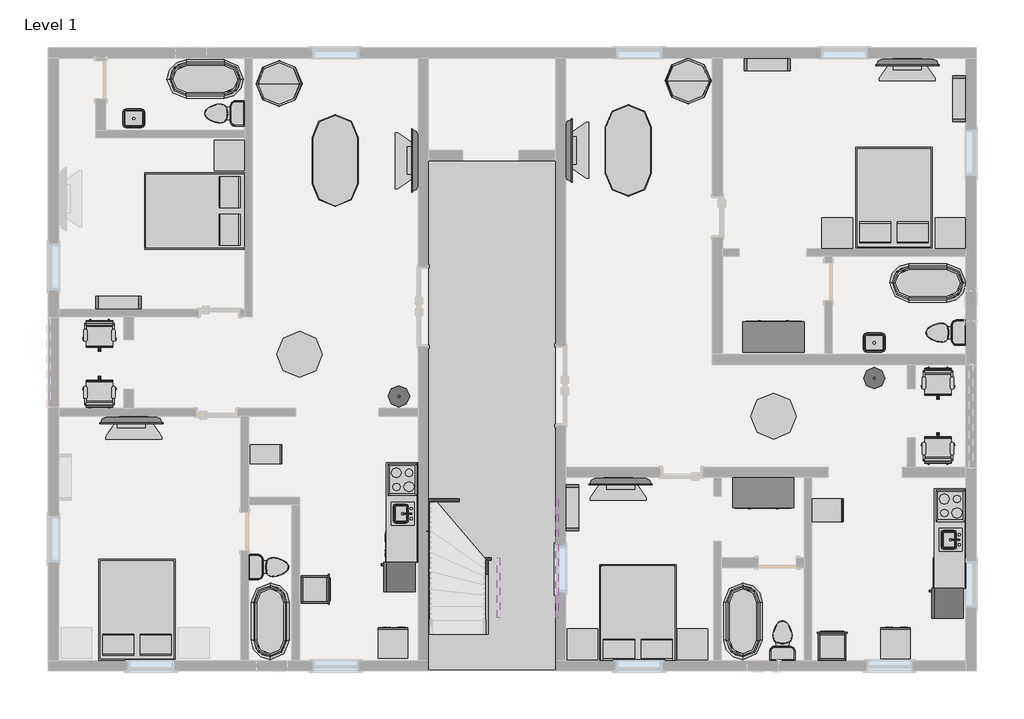
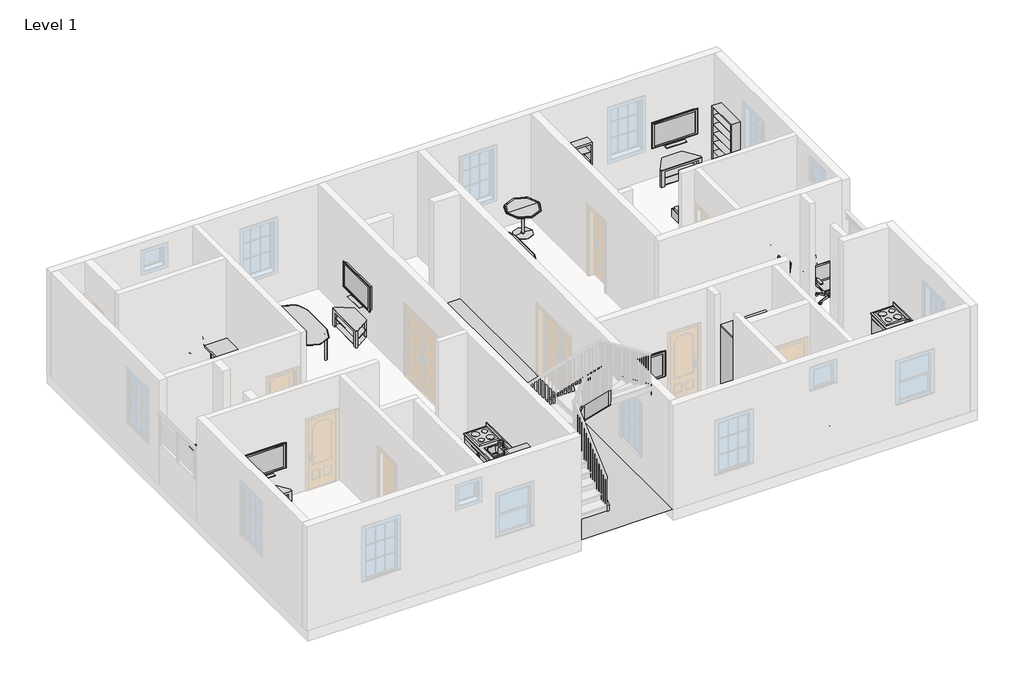
# One storey, part 4 of 4: 37 furniture elements, 15 proxies, 14 flow terminals, 8 members.
"""IFC4 building model written with IfcOpenShell, lengths in millimetres."""

from ifc_helpers import new_model, si_unit, frame, origin, place, context, project, spatial, polyline, outline, extrude, triangles, transform, mapped, element, save
from components import proxy_db4bb64d, proxy_7e1014cc, proxy_a6faaae8, proxy_53e5fb40, proxy_45b28599, kitchenette_medium_kitchenette_medium_844211aa, proxy_8b8c2dc4, proxy_c523a7b7, flow_terminal_871c2e40, flow_terminal_d49f872f, flow_terminal_62a433f7, toilet_domestic_3d_toilet_domestic_3d_f7549cf7, toilet_domestic_3d_toilet_domestic_3d_183bbd19, flow_terminal_b374fae2, furniture_1d2926bd, chair_task_arms_chair_task_arms_fa5a08ef, furniture_c6510c7c, furniture_9fa109b2, furniture_417d203a, furniture_fdf74506, tv_stand_tv_stand_6ce107e5, furniture_2c34a4f9, furniture_905aceb5, furniture_5bc9ed15, furniture_c80d6d9c

model = new_model("IFC4")

# Units and contexts
model_context = context("Model", 3, world=origin())
ifc_project = project(units=[si_unit("LENGTHUNIT", "METRE", prefix="MILLI")], contexts=[model_context])

# Site, building, storey
site = spatial("IfcSite", under=ifc_project)
building = spatial("IfcBuilding", under=site)
storey = spatial("IfcBuildingStorey", under=building, Name="Level 1", Elevation=0.0)

# Proxies
placement = place(None, origin())
element("IfcBuildingElementProxy", 1, Name="Building Element Proxy", at=placement, inside=storey, context=model_context, shape_type="Tessellation", body=[
    triangles([(-9093.3809967, 498.3923258, 0.0), (-6502.5809967, 498.3923258, 0.0), (-9093.3809967, 10671.0928345, 0.0), (-6502.5809967, 10671.0928345, 0.0)], [[3, 1, 4], [2, 4, 1]], closed=False),
])
proxy_shape = proxy_db4bb64d(model_context)
element("IfcBuildingElementProxy", 2, Name="15\" x 24\" x 34 1/2\"", ObjectType="15\" x 24\" x 34 1/2\"", at=placement, inside=storey, context=model_context, shape_type="MappedRepresentation", body=[
    mapped(proxy_shape, transform((-12040.0313324, 4522.9748669, 0.0), x_axis=(0.0, 1.000000000000001, 0.0), y_axis=(-1.000000000000001, 0.0, 0.0), z_axis=(0.0, 0.0, 1.0))),
])
proxy_2_shape = proxy_7e1014cc(model_context)
element("IfcBuildingElementProxy", 3, Name="18\" x 24\" x 34 1/2\"", ObjectType="18\" x 24\" x 34 1/2\"", at=placement, inside=storey, context=model_context, shape_type="MappedRepresentation", body=[
    mapped(proxy_2_shape, transform((-851.3313324, 3367.2748669, 0.0), x_axis=(0.0, 1.000000000000001, 0.0), y_axis=(-1.000000000000001, 0.0, 0.0), z_axis=(0.0, 0.0, 1.0))),
])
proxy_3_shape = proxy_a6faaae8(model_context)
element("IfcBuildingElementProxy", 4, Name="Cook Top-4 Unit2 : 22\" x 20\"", ObjectType="Cook Top-4 Unit2 : 22\" x 20\"", at=placement, inside=storey, context=model_context, shape_type="MappedRepresentation", body=[
    mapped(proxy_3_shape, transform((-9575.9808972, 4282.9923354, 0.0), x_axis=(0.0, -1.0000000000000004, 0.0), y_axis=(1.0000000000000004, 0.0, 0.0), z_axis=(0.0, 0.0, 1.0))),
])
element("IfcBuildingElementProxy", 5, Name="Cook Top-4 Unit2 : 22\" x 20\"", ObjectType="Cook Top-4 Unit2 : 22\" x 20\"", at=placement, inside=storey, context=model_context, shape_type="MappedRepresentation", body=[
    mapped(proxy_3_shape, transform((1346.0191028, 3762.2923354, 0.0), x_axis=(0.0, -1.0, 0.0), y_axis=(1.0, 0.0, 0.0), z_axis=(0.0, 0.0, 1.0))),
])
proxy_4_shape = proxy_53e5fb40(model_context)
element("IfcBuildingElementProxy", 6, Name="Dishwasher : 23\" x 23 11/16\" x 33 1/2\"", ObjectType="Dishwasher : 23\" x 23 11/16\" x 33 1/2\"", at=placement, inside=storey, context=model_context, shape_type="MappedRepresentation", body=[
    mapped(proxy_4_shape, transform((-9398.1808972, 1285.7923354, 0.0), x_axis=(-1.0000000000000013, 0.0, 0.0), y_axis=(0.0, -1.0000000000000013, 0.0), z_axis=(0.0, 0.0, 1.0))),
])
element("IfcBuildingElementProxy", 7, Name="Dishwasher : 23\" x 23 11/16\" x 33 1/2\"", ObjectType="Dishwasher : 23\" x 23 11/16\" x 33 1/2\"", at=placement, inside=storey, context=model_context, shape_type="MappedRepresentation", body=[
    mapped(proxy_4_shape, transform((613.9311676, 1284.4748669, 0.0), x_axis=(-1.0000000000000004, 0.0, 0.0), y_axis=(0.0, -1.0000000000000004, 0.0), z_axis=(0.0, 0.0, 1.0))),
])
proxy_5_shape = proxy_45b28599(model_context)
element("IfcBuildingElementProxy", 8, Name="Dishwasher : 24\" x 24\" x 34\"", ObjectType="Dishwasher : 24\" x 24\" x 34\"", at=placement, inside=storey, context=model_context, shape_type="MappedRepresentation", body=[
    mapped(proxy_5_shape, transform((-9867.830462, 3331.8098039, 0.0), x_axis=(0.0, -1.0000000000000004, 0.0), y_axis=(1.0000000000000004, 0.0, 0.0), z_axis=(0.0, 0.0, 1.0))),
])
element("IfcBuildingElementProxy", 9, Name="Dishwasher : 24\" x 24\" x 34\"", ObjectType="Dishwasher : 24\" x 24\" x 34\"", at=placement, inside=storey, context=model_context, shape_type="MappedRepresentation", body=[
    mapped(proxy_5_shape, transform((1054.169538, 2811.1098039, 0.0), x_axis=(0.0, -1.0, 0.0), y_axis=(1.0, 0.0, 0.0), z_axis=(0.0, 0.0, 1.0))),
])
kitchenette_medium_kitchenette_medium_shape = kitchenette_medium_kitchenette_medium_844211aa(model_context)
element("IfcBuildingElementProxy", 10, Name="Kitchenette - Medium : Kitchenette - Medium", ObjectType="Kitchenette - Medium : Kitchenette - Medium", at=placement, inside=storey, context=model_context, shape_type="MappedRepresentation", body=[
    mapped(kitchenette_medium_kitchenette_medium_shape, transform((-9271.1808972, 3958.8300403, 0.0), x_axis=(0.0, -1.0000000000000004, 0.0), y_axis=(1.0000000000000004, 0.0, 0.0), z_axis=(0.0, 0.0, 1.0))),
])
element("IfcBuildingElementProxy", 11, Name="Kitchenette - Medium : Kitchenette - Medium", ObjectType="Kitchenette - Medium : Kitchenette - Medium", at=placement, inside=storey, context=model_context, shape_type="MappedRepresentation", body=[
    mapped(kitchenette_medium_kitchenette_medium_shape, transform((1650.8191028, 3438.1300403, 0.0), x_axis=(0.0, -1.0, 0.0), y_axis=(1.0, 0.0, 0.0), z_axis=(0.0, 0.0, 1.0))),
])
proxy_6_shape = proxy_8b8c2dc4(model_context)
element("IfcBuildingElementProxy", 12, Name="Oven Double-Built-in : 21 1/2\" x 39 1/4\" x 21\"", ObjectType="Oven Double-Built-in : 21 1/2\" x 39 1/4\" x 21\"", at=placement, inside=storey, context=model_context, shape_type="MappedRepresentation", body=[
    mapped(proxy_6_shape, transform((-1051.3558245, 1096.6581944, 0.0), x_axis=(-1.0000000000000002, 0.0, 0.0), y_axis=(0.0, -1.0000000000000002, 0.0), z_axis=(0.0, 0.0, 1.0))),
])
element("IfcBuildingElementProxy", 13, Name="Oven Double-Built-in : 21 1/2\" x 39 1/4\" x 21\"", ObjectType="Oven Double-Built-in : 21 1/2\" x 39 1/4\" x 21\"", at=placement, inside=storey, context=model_context, shape_type="MappedRepresentation", body=[
    mapped(proxy_6_shape, transform((-11187.5150383, 2133.7672627, 0.0), x_axis=(0.0, 1.0000000000000002, 0.0), y_axis=(-1.0000000000000002, 0.0, 0.0), z_axis=(0.0, 0.0, 1.0))),
])
proxy_7_shape = proxy_c523a7b7(model_context)
element("IfcBuildingElementProxy", 14, Name="Refrigerator : 24\" x 25\" LH", ObjectType="Refrigerator : 24\" x 25\" LH", at=placement, inside=storey, context=model_context, shape_type="MappedRepresentation", body=[
    mapped(proxy_7_shape, transform((-9621.6298687, 2346.2423354, 0.0), x_axis=(0.0, -1.0000000000000004, 0.0), y_axis=(1.0000000000000004, 0.0, 0.0), z_axis=(0.0, 0.0, 1.0))),
])
element("IfcBuildingElementProxy", 15, Name="Refrigerator : 24\" x 25\" LH", ObjectType="Refrigerator : 24\" x 25\" LH", at=placement, inside=storey, context=model_context, shape_type="MappedRepresentation", body=[
    mapped(proxy_7_shape, transform((1300.3701313, 1825.5423354, 0.0), x_axis=(0.0, -1.0, 0.0), y_axis=(1.0, 0.0, 0.0), z_axis=(0.0, 0.0, 1.0))),
])

# Flow terminals
flow_terminal_shape = flow_terminal_871c2e40(model_context)
element("IfcFlowTerminal", 16, ObjectType="Sink Kitchen-Island : 18\" x 18\"", at=placement, inside=storey, context=model_context, shape_type="MappedRepresentation", body=[
    mapped(flow_terminal_shape, transform((-9578.3262983, 3625.581576, -14.4), x_axis=(0.0, -1.0000000000000004, 0.0), y_axis=(1.0000000000000004, 0.0, 0.0), z_axis=(0.0, 0.0, 1.0))),
])
element("IfcFlowTerminal", 17, ObjectType="Sink Kitchen-Island : 18\" x 18\"", at=placement, inside=storey, context=model_context, shape_type="MappedRepresentation", body=[
    mapped(flow_terminal_shape, transform((1343.6737017, 3104.881576, -14.4), x_axis=(0.0, -1.0, 0.0), y_axis=(1.0, 0.0, 0.0), z_axis=(0.0, 0.0, 1.0))),
])
flow_terminal_2_shape = flow_terminal_d49f872f(model_context)
element("IfcFlowTerminal", 18, ObjectType="Sink Vanity-Round : 19\" x 19\"", at=placement, inside=storey, context=model_context, shape_type="MappedRepresentation", body=[
    mapped(flow_terminal_2_shape, transform((-274.6326378, 6226.604818, 609.6), x_axis=(1.0, 0.0, 0.0), y_axis=(0.0, 1.0, 0.0), z_axis=(0.0, 0.0, 1.0))),
])
element("IfcFlowTerminal", 19, ObjectType="Sink Vanity-Round : 19\" x 19\"", at=placement, inside=storey, context=model_context, shape_type="MappedRepresentation", body=[
    mapped(flow_terminal_2_shape, transform((-9555.5291566, 6031.4364541, 609.6), x_axis=(-1.0000000000000004, 0.0, 0.0), y_axis=(0.0, -1.0000000000000004, 0.0), z_axis=(0.0, 0.0, 1.0))),
])
flow_terminal_3_shape = flow_terminal_62a433f7(model_context)
element("IfcFlowTerminal", 20, ObjectType="Sink Vanity-Square : 20\" x 18\"", at=placement, inside=storey, context=model_context, shape_type="MappedRepresentation", body=[
    mapped(flow_terminal_3_shape, transform((-162.2916566, 6965.0377365, 609.6), x_axis=(-1.0000000000000004, 0.0, 0.0), y_axis=(0.0, -1.0000000000000004, 0.0), z_axis=(0.0, 0.0, 1.0))),
])
element("IfcFlowTerminal", 21, ObjectType="Sink Vanity-Square : 20\" x 18\"", at=placement, inside=storey, context=model_context, shape_type="MappedRepresentation", body=[
    mapped(flow_terminal_3_shape, transform((-14919.6916566, 11435.4377365, 609.6), x_axis=(-1.0, 0.0, 0.0), y_axis=(0.0, -1.0, 0.0), z_axis=(0.0, 0.0, 1.0))),
])
toilet_domestic_3d_toilet_domestic_3d_shape = toilet_domestic_3d_toilet_domestic_3d_f7549cf7(model_context)
toilet_domestic_3d_toilet_domestic_3d_2_shape = toilet_domestic_3d_toilet_domestic_3d_183bbd19(model_context)
element("IfcFlowTerminal", 22, ObjectType="Toilet-Domestic-3D : Toilet-Domestic-3D", at=placement, inside=storey, context=model_context, shape_type="MappedRepresentation", body=[
    mapped(toilet_domestic_3d_toilet_domestic_3d_shape, transform((-12154.6848699, 2543.0923354, 0.0), x_axis=(0.0, 1.0000000000000002, 0.0), y_axis=(-1.0000000000000002, 0.0, 0.0), z_axis=(0.0, 0.0, 1.0))),
    mapped(toilet_domestic_3d_toilet_domestic_3d_2_shape, transform((-12154.6848699, 2543.0923354, 0.0), x_axis=(0.0, 1.0000000000000002, 0.0), y_axis=(-1.0000000000000002, 0.0, 0.0), z_axis=(0.0, 0.0, 1.0))),
])
element("IfcFlowTerminal", 23, ObjectType="Toilet-Domestic-3D : Toilet-Domestic-3D", at=placement, inside=storey, context=model_context, shape_type="MappedRepresentation", body=[
    mapped(toilet_domestic_3d_toilet_domestic_3d_shape, transform((-2006.7808972, 1170.8883628, 0.0), x_axis=(-1.0000000000000004, 0.0, 0.0), y_axis=(0.0, -1.0000000000000004, 0.0), z_axis=(0.0, 0.0, 1.0))),
    mapped(toilet_domestic_3d_toilet_domestic_3d_2_shape, transform((-2006.7808972, 1170.8883628, 0.0), x_axis=(-1.0000000000000004, 0.0, 0.0), y_axis=(0.0, -1.0000000000000004, 0.0), z_axis=(0.0, 0.0, 1.0))),
])
element("IfcFlowTerminal", 24, ObjectType="Toilet-Domestic-3D : Toilet-Domestic-3D", at=placement, inside=storey, context=model_context, shape_type="MappedRepresentation", body=[
    mapped(toilet_domestic_3d_toilet_domestic_3d_shape, transform((1156.1230754, 7216.6923354, 0.0), x_axis=(0.0, -1.0000000000000002, 0.0), y_axis=(1.0000000000000002, 0.0, 0.0), z_axis=(0.0, 0.0, 1.0))),
    mapped(toilet_domestic_3d_toilet_domestic_3d_2_shape, transform((1156.1230754, 7216.6923354, 0.0), x_axis=(0.0, -1.0000000000000002, 0.0), y_axis=(1.0000000000000002, 0.0, 0.0), z_axis=(0.0, 0.0, 1.0))),
])
element("IfcFlowTerminal", 25, ObjectType="Toilet-Domestic-3D : Toilet-Domestic-3D", at=placement, inside=storey, context=model_context, shape_type="MappedRepresentation", body=[
    mapped(toilet_domestic_3d_toilet_domestic_3d_shape, transform((-13220.2769246, 11585.4923354, 0.0), x_axis=(0.0, -1.0, 0.0), y_axis=(1.0, 0.0, 0.0), z_axis=(0.0, 0.0, 1.0))),
    mapped(toilet_domestic_3d_toilet_domestic_3d_2_shape, transform((-13220.2769246, 11585.4923354, 0.0), x_axis=(0.0, -1.0, 0.0), y_axis=(1.0, 0.0, 0.0), z_axis=(0.0, 0.0, 1.0))),
])
flow_terminal_4_shape = flow_terminal_b374fae2(model_context)
element("IfcFlowTerminal", 26, ObjectType="Tub-Free Standing-3D : 30\" x 60\"", at=placement, inside=storey, context=model_context, shape_type="MappedRepresentation", body=[
    mapped(flow_terminal_4_shape, transform((888.8191028, 8207.2923354, 0.0), x_axis=(0.0, -1.0000000000000002, 0.0), y_axis=(1.0000000000000002, 0.0, 0.0), z_axis=(0.0, 0.0, 1.0))),
])
element("IfcFlowTerminal", 27, ObjectType="Tub-Free Standing-3D : 30\" x 60\"", at=placement, inside=storey, context=model_context, shape_type="MappedRepresentation", body=[
    mapped(flow_terminal_4_shape, transform((-2794.1808972, 1463.5923354, 0.0), x_axis=(-1.0000000000000004, 0.0, 0.0), y_axis=(0.0, -1.0000000000000004, 0.0), z_axis=(0.0, 0.0, 1.0))),
])
element("IfcFlowTerminal", 28, ObjectType="Tub-Free Standing-3D : 30\" x 60\"", at=placement, inside=storey, context=model_context, shape_type="MappedRepresentation", body=[
    mapped(flow_terminal_4_shape, transform((-13512.9808972, 12271.2923354, 0.0), x_axis=(0.0, -1.0, 0.0), y_axis=(1.0, 0.0, 0.0), z_axis=(0.0, 0.0, 1.0))),
])
element("IfcFlowTerminal", 29, ObjectType="Tub-Free Standing-3D : 30\" x 60\"", at=placement, inside=storey, context=model_context, shape_type="MappedRepresentation", body=[
    mapped(flow_terminal_4_shape, transform((-12217.5808972, 1463.5923354, 0.0), x_axis=(-0.9999999999999998, 0.0, 0.0), y_axis=(0.0, -0.9999999999999998, 0.0), z_axis=(0.0, 0.0, 1.0))),
])

# Furniture
furniture_shape = furniture_1d2926bd(model_context)
element("IfcFurniture", 30, ObjectType="Bed-Box : Queen 60\" x 79\"", at=placement, inside=storey, context=model_context, shape_type="MappedRepresentation", body=[
    mapped(furniture_shape, transform((-13481.751389, 9981.5447944, 0.0), x_axis=(0.0, -1.0000000000000002, 0.0), y_axis=(1.0000000000000002, 0.0, 0.0), z_axis=(0.0, 0.0, 1.0))),
])
element("IfcFurniture", 31, ObjectType="Bed-Box : Queen 60\" x 79\"", at=placement, inside=storey, context=model_context, shape_type="MappedRepresentation", body=[
    mapped(furniture_shape, transform((-14532.7284382, 1457.7628272, 0.0), x_axis=(-0.9999999999999998, 0.0, 0.0), y_axis=(0.0, -0.9999999999999998, 0.0), z_axis=(0.0, 0.0, 1.0))),
])
element("IfcFurniture", 32, ObjectType="Bed-Box : Queen 60\" x 79\"", at=placement, inside=storey, context=model_context, shape_type="MappedRepresentation", body=[
    mapped(furniture_shape, transform((-4550.5284382, 1356.1628272, 0.0), x_axis=(-1.0, 0.0, 0.0), y_axis=(0.0, -1.0, 0.0), z_axis=(0.0, 0.0, 1.0))),
])
element("IfcFurniture", 33, ObjectType="Bed-Box : Queen 60\" x 79\"", at=placement, inside=storey, context=model_context, shape_type="MappedRepresentation", body=[
    mapped(furniture_shape, transform((554.8715618, 9674.6628272, 0.0), x_axis=(-1.0, 0.0, 0.0), y_axis=(0.0, -1.0, 0.0), z_axis=(0.0, 0.0, 1.0))),
])
chair_task_arms_chair_task_arms_shape = chair_task_arms_chair_task_arms_fa5a08ef(model_context)
element("IfcFurniture", 34, ObjectType="Chair-Task Arms : Chair-Task Arms", at=placement, inside=storey, context=model_context, shape_type="MappedRepresentation", body=[
    mapped(chair_task_arms_chair_task_arms_shape, transform((-15762.1717169, 5978.5464338, 0.0), x_axis=(1.0, 0.0, 0.0), y_axis=(0.0, 1.0, 0.0), z_axis=(0.0, 0.0, 1.0))),
])
element("IfcFurniture", 35, ObjectType="Chair-Task Arms : Chair-Task Arms", at=placement, inside=storey, context=model_context, shape_type="MappedRepresentation", body=[
    mapped(chair_task_arms_chair_task_arms_shape, transform((-15480.1900775, 7210.2382371, 0.0), x_axis=(-1.0000000000000004, 0.0, 0.0), y_axis=(0.0, -1.0000000000000004, 0.0), z_axis=(0.0, 0.0, 1.0))),
])
element("IfcFurniture", 36, ObjectType="Chair-Task Arms : Chair-Task Arms", at=placement, inside=storey, context=model_context, shape_type="MappedRepresentation", body=[
    mapped(chair_task_arms_chair_task_arms_shape, transform((1233.0099225, 6257.7382371, 0.0), x_axis=(-1.0, 0.0, 0.0), y_axis=(0.0, -1.0, 0.0), z_axis=(0.0, 0.0, 1.0))),
])
element("IfcFurniture", 37, ObjectType="Chair-Task Arms : Chair-Task Arms", at=placement, inside=storey, context=model_context, shape_type="MappedRepresentation", body=[
    mapped(chair_task_arms_chair_task_arms_shape, transform((951.0282831, 4860.9464338, 0.0), x_axis=(1.0000000000000002, 0.0, 0.0), y_axis=(0.0, 1.0000000000000002, 0.0), z_axis=(0.0, 0.0, 1.0))),
])
furniture_2_shape = furniture_c6510c7c(model_context)
element("IfcFurniture", 38, ObjectType="Counter Top w Sink Hole : 24\" Depth", at=placement, inside=storey, context=model_context, shape_type="MappedRepresentation", body=[
    mapped(furniture_2_shape, transform((-9271.1808972, 3425.4300403, -14.4), x_axis=(0.0, -1.0000000000000004, 0.0), y_axis=(1.0000000000000004, 0.0, 0.0), z_axis=(0.0, 0.0, 1.0))),
])
element("IfcFurniture", 39, ObjectType="Counter Top w Sink Hole : 24\" Depth", at=placement, inside=storey, context=model_context, shape_type="MappedRepresentation", body=[
    mapped(furniture_2_shape, transform((1650.8191028, 2904.7300403, -14.4), x_axis=(0.0, -1.0, 0.0), y_axis=(1.0, 0.0, 0.0), z_axis=(0.0, 0.0, 1.0))),
])
furniture_3_shape = furniture_9fa109b2(model_context)
element("IfcFurniture", 40, ObjectType="Dresser : 48\" x 72\" x 24\"", at=placement, inside=storey, context=model_context, shape_type="MappedRepresentation", body=[
    mapped(furniture_3_shape, transform((-2453.774157, 6764.6293813, 0.0), x_axis=(-1.0000000000000004, 0.0, 0.0), y_axis=(0.0, -1.0000000000000004, 0.0), z_axis=(0.0, 0.0, 1.0))),
])
element("IfcFurniture", 41, ObjectType="Dresser : 48\" x 72\" x 24\"", at=placement, inside=storey, context=model_context, shape_type="MappedRepresentation", body=[
    mapped(furniture_3_shape, transform((-2118.5876374, 4392.1552895, 0.0), x_axis=(1.0, 0.0, 0.0), y_axis=(0.0, 1.0, 0.0), z_axis=(0.0, 0.0, 1.0))),
])
furniture_4_shape = furniture_417d203a(model_context)
element("IfcFurniture", 42, ObjectType="Shelving : 36\" x 10\" x 72\"", at=placement, inside=storey, context=model_context, shape_type="MappedRepresentation", body=[
    mapped(furniture_4_shape, transform((-15240.1808972, 8118.3923354, 0.0), x_axis=(1.0, 0.0, 0.0), y_axis=(0.0, 1.0, 0.0), z_axis=(0.0, 0.0, 1.0))),
])
element("IfcFurniture", 43, ObjectType="Shelving : 36\" x 10\" x 72\"", at=placement, inside=storey, context=model_context, shape_type="MappedRepresentation", body=[
    mapped(furniture_4_shape, transform((-6502.5808972, 3724.1923354, 0.0), x_axis=(0.0, 1.0000000000000002, 0.0), y_axis=(-1.0000000000000002, 0.0, 0.0), z_axis=(0.0, 0.0, 1.0))),
])
element("IfcFurniture", 44, ObjectType="Shelving : 36\" x 10\" x 72\"", at=placement, inside=storey, context=model_context, shape_type="MappedRepresentation", body=[
    mapped(furniture_4_shape, transform((-2311.5808972, 12258.5923354, 0.0), x_axis=(-1.0000000000000004, 0.0, 0.0), y_axis=(0.0, -1.0000000000000004, 0.0), z_axis=(0.0, 0.0, 1.0))),
])
element("IfcFurniture", 45, ObjectType="Shelving : 36\" x 10\" x 72\"", at=placement, inside=storey, context=model_context, shape_type="MappedRepresentation", body=[
    mapped(furniture_4_shape, transform((1815.9191028, 11877.5923354, 0.0), x_axis=(0.0, -1.0000000000000002, 0.0), y_axis=(1.0000000000000002, 0.0, 0.0), z_axis=(0.0, 0.0, 1.0))),
])
furniture_5_shape = furniture_fdf74506(model_context)
element("IfcFurniture", 46, ObjectType="TV - Flat Screen : 50\"", at=placement, inside=storey, context=model_context, shape_type="MappedRepresentation", body=[
    mapped(furniture_5_shape, transform((-14982.2363831, 5470.9664028, 914.4), x_axis=(1.0, 0.0, 0.0), y_axis=(0.0, 1.0, 0.0), z_axis=(0.0, 0.0, 1.0))),
])
element("IfcFurniture", 47, ObjectType="TV - Flat Screen : 50\"", at=placement, inside=storey, context=model_context, shape_type="MappedRepresentation", body=[
    mapped(furniture_5_shape, transform((-5228.6363831, 4251.4680978, 914.4), x_axis=(1.0, 0.0, 0.0), y_axis=(0.0, 1.0, 0.0), z_axis=(0.0, 0.0, 1.0))),
])
element("IfcFurniture", 48, ObjectType="TV - Flat Screen : 50\"", at=placement, inside=storey, context=model_context, shape_type="MappedRepresentation", body=[
    mapped(furniture_5_shape, transform((486.3636169, 12605.0152005, 914.4), x_axis=(1.0, 0.0, 0.0), y_axis=(0.0, 1.0, 0.0), z_axis=(0.0, 0.0, 1.0))),
])
element("IfcFurniture", 49, ObjectType="TV - Flat Screen : 50\"", at=placement, inside=storey, context=model_context, shape_type="MappedRepresentation", body=[
    mapped(furniture_5_shape, transform((-9329.7195209, 10641.7478213, 914.4), x_axis=(0.0, -0.9999999999999998, 0.0), y_axis=(0.9999999999999998, 0.0, 0.0), z_axis=(0.0, 0.0, 1.0))),
])
element("IfcFurniture", 50, ObjectType="TV - Flat Screen : 50\"", at=placement, inside=storey, context=model_context, shape_type="MappedRepresentation", body=[
    mapped(furniture_5_shape, transform((-6266.2422736, 10852.8368496, 914.4), x_axis=(0.0, 1.0000000000000004, 0.0), y_axis=(-1.0000000000000004, 0.0, 0.0), z_axis=(0.0, 0.0, 1.0))),
])
tv_stand_tv_stand_shape = tv_stand_tv_stand_6ce107e5(model_context)
element("IfcFurniture", 51, ObjectType="TV Stand : TV Stand", at=placement, inside=storey, context=model_context, shape_type="MappedRepresentation", body=[
    mapped(tv_stand_tv_stand_shape, transform((357.2311007, 12690.3923354, 0.0), x_axis=(1.0, 0.0, 0.0), y_axis=(0.0, 1.0, 0.0), z_axis=(0.0, 0.0, 1.0))),
])
element("IfcFurniture", 52, ObjectType="TV Stand : TV Stand", at=placement, inside=storey, context=model_context, shape_type="MappedRepresentation", body=[
    mapped(tv_stand_tv_stand_shape, transform((-15060.5688993, 5552.9923354, 0.0), x_axis=(1.0, 0.0, 0.0), y_axis=(0.0, 1.0, 0.0), z_axis=(0.0, 0.0, 1.0))),
])
element("IfcFurniture", 53, ObjectType="TV Stand : TV Stand", at=placement, inside=storey, context=model_context, shape_type="MappedRepresentation", body=[
    mapped(tv_stand_tv_stand_shape, transform((-5408.5688993, 4333.7923354, 0.0), x_axis=(1.0, 0.0, 0.0), y_axis=(0.0, 1.0, 0.0), z_axis=(0.0, 0.0, 1.0))),
])
element("IfcFurniture", 54, ObjectType="TV Stand : TV Stand", at=placement, inside=storey, context=model_context, shape_type="MappedRepresentation", body=[
    mapped(tv_stand_tv_stand_shape, transform((-6324.7808972, 10723.7043334, 0.0), x_axis=(0.0, 1.0, 0.0), y_axis=(-1.0, 0.0, 0.0), z_axis=(0.0, 0.0, 1.0))),
])
element("IfcFurniture", 55, ObjectType="TV Stand : TV Stand", at=placement, inside=storey, context=model_context, shape_type="MappedRepresentation", body=[
    mapped(tv_stand_tv_stand_shape, transform((-9271.1808972, 10770.8803375, 0.0), x_axis=(0.0, -1.0000000000000002, 0.0), y_axis=(1.0000000000000002, 0.0, 0.0), z_axis=(0.0, 0.0, 1.0))),
])
furniture_6_shape = furniture_2c34a4f9(model_context)
element("IfcFurniture", 56, ObjectType="Table-Dining Oval : 36\" x 72\"", at=placement, inside=storey, context=model_context, shape_type="MappedRepresentation", body=[
    mapped(furniture_6_shape, transform((-5438.2792579, 11250.7120076, 0.0), x_axis=(0.0, 1.0, 0.0), y_axis=(-1.0, 0.0, 0.0), z_axis=(0.0, 0.0, 1.0))),
])
element("IfcFurniture", 57, ObjectType="Table-Dining Oval : 36\" x 72\"", at=placement, inside=storey, context=model_context, shape_type="MappedRepresentation", body=[
    mapped(furniture_6_shape, transform((-11280.2792579, 11047.5120076, 0.0), x_axis=(0.0, 1.0, 0.0), y_axis=(-1.0, 0.0, 0.0), z_axis=(0.0, 0.0, 1.0))),
])
furniture_7_shape = furniture_905aceb5(model_context)
element("IfcFurniture", 58, ObjectType="Table-Dining Round w Chairs : 36\" Diameter", at=placement, inside=storey, context=model_context, shape_type="MappedRepresentation", body=[
    mapped(furniture_7_shape, transform((-2288.2628644, 5737.8710239, 0.0), x_axis=(1.0, 0.0, 0.0), y_axis=(0.0, 1.0, 0.0), z_axis=(0.0, 0.0, 1.0))),
])
element("IfcFurniture", 59, ObjectType="Table-Dining Round w Chairs : 36\" Diameter", at=placement, inside=storey, context=model_context, shape_type="MappedRepresentation", body=[
    mapped(furniture_7_shape, transform((-11737.0628644, 6969.7710239, 0.0), x_axis=(1.0, 0.0, 0.0), y_axis=(0.0, 1.0, 0.0), z_axis=(0.0, 0.0, 1.0))),
])
furniture_8_shape = furniture_5bc9ed15(model_context)
element("IfcFurniture", 60, ObjectType="Table-Night Stand : 24\" x 24\" x 30\"", at=placement, inside=storey, context=model_context, shape_type="MappedRepresentation", body=[
    mapped(furniture_8_shape, transform((1037.4854725, 8893.0923354, 0.0), x_axis=(1.0, 0.0, 0.0), y_axis=(0.0, 1.0, 0.0), z_axis=(0.0, 0.0, 1.0))),
])
element("IfcFurniture", 61, ObjectType="Table-Night Stand : 24\" x 24\" x 30\"", at=placement, inside=storey, context=model_context, shape_type="MappedRepresentation", body=[
    mapped(furniture_8_shape, transform((-1223.1145275, 8893.0923354, 0.0), x_axis=(1.0, 0.0, 0.0), y_axis=(0.0, 1.0, 0.0), z_axis=(0.0, 0.0, 1.0))),
])
element("IfcFurniture", 62, ObjectType="Table-Night Stand : 24\" x 24\" x 30\"", at=placement, inside=storey, context=model_context, shape_type="MappedRepresentation", body=[
    mapped(furniture_8_shape, transform((-6303.1145275, 701.5923354, 0.0), x_axis=(1.0, 0.0, 0.0), y_axis=(0.0, 1.0, 0.0), z_axis=(0.0, 0.0, 1.0))),
])
element("IfcFurniture", 63, ObjectType="Table-Night Stand : 24\" x 24\" x 30\"", at=placement, inside=storey, context=model_context, shape_type="MappedRepresentation", body=[
    mapped(furniture_8_shape, transform((-4106.0145275, 701.5923354, 0.0), x_axis=(1.0, 0.0, 0.0), y_axis=(0.0, 1.0, 0.0), z_axis=(0.0, 0.0, 1.0))),
])
element("IfcFurniture", 64, ObjectType="Table-Night Stand : 24\" x 24\" x 30\"", at=placement, inside=storey, context=model_context, shape_type="MappedRepresentation", body=[
    mapped(furniture_8_shape, transform((-13338.9145275, 10442.4923354, 0.0), x_axis=(1.0, 0.0, 0.0), y_axis=(0.0, 1.0, 0.0), z_axis=(0.0, 0.0, 1.0))),
])
furniture_9_shape = furniture_c80d6d9c(model_context)
element("IfcFurniture", 65, ObjectType="Table-Round : 36\" Diameter", at=placement, inside=storey, context=model_context, shape_type="MappedRepresentation", body=[
    mapped(furniture_9_shape, transform((-3886.3808972, 12233.1923354, 0.0), x_axis=(1.0, 0.0, 0.0), y_axis=(0.0, 1.0, 0.0), z_axis=(0.0, 0.0, 1.0))),
])
element("IfcFurniture", 66, ObjectType="Table-Round : 36\" Diameter", at=placement, inside=storey, context=model_context, shape_type="MappedRepresentation", body=[
    mapped(furniture_9_shape, transform((-12039.7808972, 12182.3923354, 0.0), x_axis=(1.0, 0.0, 0.0), y_axis=(0.0, 1.0, 0.0), z_axis=(0.0, 0.0, 1.0))),
])

# Members
element("IfcMember", 67, ObjectType="Stringer - 2\" Width", at=placement, inside=storey, context=model_context, shape_type="SweptSolid", body=[
    extrude(outline(polyline([(1205.8606436, 0.0), (1205.8606436, 239.0560697), (3583.7706661, 1355.0732539), (3583.7706661, 1018.373708), (1413.9106664, 0.0), (1205.8606436, 0.0)])), frame((-9093.3808972, 0.0, 0.0), z_axis=(1.0, 0.0, 0.0), x_axis=(0.0, 1.0, 0.0)), (0.0, 0.0, 1.0), 50.8),
])
element("IfcMember", 68, ObjectType="Stringer - 2\" Width", at=placement, inside=storey, context=model_context, shape_type="SweptSolid", body=[
    extrude(outline(polyline([(-9042.5808972, 3583.7706661), (-9093.3808972, 3583.7706661), (-9093.3808972, 3851.1923354), (-9042.5808972, 3851.1923354), (-9042.5808972, 3583.7706661)])), frame((0.0, 0.0, 1018.373708), z_axis=(0.0, 0.0, 1.0), x_axis=(1.0, 0.0, 0.0)), (0.0, 0.0, 1.0), 336.6995459),
])
element("IfcMember", 69, ObjectType="Stringer - 2\" Width", at=placement, inside=storey, context=model_context, shape_type="SweptSolid", body=[
    extrude(outline(polyline([(1339.5001803, -9093.3808972), (1050.2732539, -9093.3808972), (1050.2732539, -8938.52328), (1789.2408513, -6527.9808972), (2116.9383072, -6527.9808972), (2116.9383072, -6557.3460815), (1339.5001803, -9093.3808972)])), frame((0.0, 3851.1923354, 0.0), z_axis=(0.0, 1.0, 0.0), x_axis=(0.0, 0.0, 1.0)), (0.0, 0.0, 1.0), 50.8),
])
element("IfcMember", 70, ObjectType="Stringer - 2\" Width", at=placement, inside=storey, context=model_context, shape_type="SweptSolid", body=[
    extrude(outline(polyline([(-6527.9808972, 3901.9923354), (-6477.1808972, 3901.9923354), (-6477.1808972, 3591.7070571), (-6527.9808972, 3591.7070571), (-6527.9808972, 3901.9923354)])), frame((0.0, 0.0, 1798.1377702), z_axis=(0.0, 0.0, 1.0), x_axis=(1.0, 0.0, 0.0)), (0.0, 0.0, 1.0), 318.800537),
])
element("IfcMember", 71, ObjectType="Stringer - 2\" Width", at=placement, inside=storey, context=model_context, shape_type="SweptSolid", body=[
    extrude(outline(polyline([(3591.7070571, 2116.9383072), (3591.7070571, 1798.1377702), (1529.5899254, 2705.2958866), (1529.5899254, 3024.0964236), (3591.7070571, 2116.9383072)])), frame((-6527.9808972, 0.0, 0.0), z_axis=(1.0, 0.0, 0.0), x_axis=(0.0, 1.0, 0.0)), (0.0, 0.0, 1.0), 50.8),
])
element("IfcMember", 72, ObjectType="Stringer - 2\" Width", at=placement, inside=storey, context=model_context, shape_type="SweptSolid", body=[
    extrude(outline(polyline([(1205.8606436, 0.0), (1205.8606436, 167.5499862), (2682.7923354, 1453.6547636), (2682.7923354, 1049.4890458), (1477.58444, 0.0), (1205.8606436, 0.0)])), frame((-7924.9808972, 0.0, 0.0), z_axis=(1.0, 0.0, 0.0), x_axis=(0.0, 1.0, 0.0)), (0.0, 0.0, 1.0), 50.8),
])
element("IfcMember", 73, ObjectType="Stringer - 2\" Width", at=placement, inside=storey, context=model_context, shape_type="SweptSolid", body=[
    extrude(outline(polyline([(1700.8855831, -7924.9808972), (1093.7254334, -7924.9808972), (1093.7254334, -7856.1870068), (1462.0009709, -7696.3808972), (2072.0814189, -7696.3808972), (2072.0814189, -7763.9075802), (1700.8855831, -7924.9808972)])), frame((0.0, 2682.7923354, 0.0), z_axis=(0.0, 1.0, 0.0), x_axis=(0.0, 0.0, 1.0)), (0.0, 0.0, 1.0), 50.8),
])
element("IfcMember", 74, ObjectType="Stringer - 2\" Width", at=placement, inside=storey, context=model_context, shape_type="SweptSolid", body=[
    extrude(outline(polyline([(2733.5923354, 2072.0814189), (2733.5923354, 1648.7996171), (1529.5899254, 2808.98745), (1529.5899254, 3232.2692517), (2733.5923354, 2072.0814189)])), frame((-7696.3808972, 0.0, 0.0), z_axis=(1.0, 0.0, 0.0), x_axis=(0.0, 1.0, 0.0)), (0.0, 0.0, 1.0), 50.8),
])

save(model, "model.ifc")

# Revit data of these elements
# Type "15\" x 24\" x 34 1/2\""
#   Label = "T"
#   Assembly Code = "E1090400"
#   Depth = 2' - 0"
#   Height = 2' - 10 1/2"
#   Width = 1' - 3"
#   Panel Face Material = Plastic, Opaque Black
#   Trach Compact. Material = Steel, Paint Finish, Ivory, Matte
#   Default Elevation = 0
# Type "18\" x 24\" x 34 1/2\""
#   Label = "T"
#   Assembly Code = "E1090400"
#   Depth = 2' - 0"
#   Height = 2' - 10 1/2"
#   Width = 1' - 6"
#   Panel Face Material = Plastic, Opaque Black
#   Trach Compact. Material = Steel, Paint Finish, Ivory, Matte
#   Default Elevation = 0
# Type "Cook Top-4 Unit2 : 22\" x 20\""
#   Depth = 1' - 8"
#   Width = 1' - 10"
#   Burner Material = Steel, Chrome Plated
#   Cooktop Material = Steel, Polished
#   Default Elevation = 0
#   Assembly Code = ""
# Type "Dishwasher : 23\" x 23 11/16\" x 33 1/2\""
#   Label = "DW"
#   Assembly Code = "E1090400"
#   Depth = 1' - 11 11/16"
#   Height = 2' - 9 1/2"
#   Width = 1' - 11"
#   Dishwasher Material = Steel, Paint Finish, Ivory, Glossy
#   Panel Face Material = Plastic, Opaque Black
#   Default Elevation = 0
# Type "Dishwasher : 24\" x 24\" x 34\""
#   Label = "DW"
#   Assembly Code = "E1090400"
#   Depth = 2' - 0"
#   Height = 2' - 10"
#   Width = 2' - 0"
#   Dishwasher Material = Steel, Paint Finish, Ivory, Glossy
#   Panel Face Material = Plastic, Opaque Black
#   Default Elevation = 0
# Type "Kitchenette - Medium : Kitchenette - Medium"
#   Assembly Code = "E1090400"
#   Counter Length = 6' - 6"
#   Cabinet Width = 4' - 6"
#   Cabinet Height = 2' - 10 1/2"
#   Cabinet Depth = 2' - 0"
#   Toe Depth = 0' - 3"
#   Toe Height = 0' - 3 1/2"
#   Cabinet Material = Cabinets
#   Door/Drawer Material = Cabinets
#   Handle Material = Cabinets - Handles
#   Default Elevation = 0
# Type "Oven Double-Built-in : 21 1/2\" x 39 1/4\" x 21\""
#   Label = "OVEN"
#   Assembly Code = "E1090400"
#   Depth = 1' - 9"
#   Height = 3' - 3 1/4"
#   Width = 1' - 9 1/2"
#   Oven Material = Metal - Stainless Steel, Polished
#   Default Elevation = 0
# Type "Refrigerator : 24\" x 25\" LH"
#   Label = "REF."
#   Assembly Code = "E1090400"
#   Depth = 2' - 0 3/4"
#   Handle = 0' - 1 1/2"
#   Height = 5' - 3 1/2"
#   Rear Clearance = 0' - 2"
#   Top Door Height = 1' - 8"
#   Width = 1' - 11 1/2"
#   Material = Steel, Paint Finish, Ivory, Glossy
#   Default Elevation = 0
# Type "Sink Kitchen-Island : 18\" x 18\""
#   Assembly Code = "D2010410"
#   Counter Height = 3' - 0"
#   Depth = 1' - 6"
#   Width = 1' - 6"
#   Faucet Material = Steel, Polished
#   Sink Material = Steel, Polished
#   Default Elevation = 0
# Type "Sink Vanity-Round : 19\" x 19\""
#   Assembly Code = "D2010400"
#   Top Of Counter = 2' - 7"
#   Basin Material = Porcelain, Linen
#   Faucet Material = Steel, Polished
#   Default Elevation = 0
# Type "Sink Vanity-Square : 20\" x 18\""
#   Assembly Code = "D2010400"
#   Counter Height = 2' - 7"
#   Depth = 1' - 6"
#   Width = 1' - 8"
#   Basin Material = Porcelain, Linen
#   Faucet Material = Steel, Polished
#   Default Elevation = 0
# Type "Toilet-Domestic-3D : Toilet-Domestic-3D"
#   Assembly Code = "D2010110"
#   Toilet - Bowl/Basin Material = Porcelain, Linen
#   Toilet - Seat Material = Laminate, Linen, Matte
#   Default Elevation = 0
# Type "Tub-Free Standing-3D : 30\" x 60\""
#   Assembly Code = "D2010110"
#   Height = 1' - 6"
#   Length = 5' - 0"
#   Width = 2' - 6"
#   Tub Material = Porcelain, Ivory
#   Default Elevation = 0
# Type "Bed-Box : Queen 60\" x 79\""
#   Assembly Code = "E2020200"
#   Length = 6' - 7"
#   Width = 5' - 0"
#   Frame Material = Birch
#   Mattress Material = Linen, White
#   Default Elevation = 0
# Type "Chair-Task Arms : Chair-Task Arms"
#   Assembly Code = "E2020200"
#   Base Material = Plastic, Opaque Black
#   Caster Material = Plastic, Opaque Black
#   Seat/Back Material = Textile - Slate Blue
#   Default Elevation = 0
# Type "Counter Top w Sink Hole : 24\" Depth"
#   Assembly Code = "C1030400"
#   Counter Thickness = 0' - 1 1/2"
#   Depth = 2' - 1"
#   Height = 3' - 0"
#   Length [instance default] = 8' - 0"
#   Sink Location [instance default] = 2' - 0"
#   Sink Location To Wall [instance default] = 0' - 6"
#   Sink Opening Depth [instance default] = 1' - 3"
#   Sink Opening Width [instance default] = 2' - 3"
#   Counter Top Material = none
#   Default Elevation = 0
# Type "Dresser : 48\" x 72\" x 24\""
#   Assembly Code = "E2020200"
#   Depth = 2' - 0"
#   Height = 6' - 0"
#   Width = 4' - 0"
#   Dresser Material = Laminate - Ivory, Glossy
#   Drawer Material = Laminate, Ivory, Matte
#   Knob Material = Cherry
#   Default Elevation = 0
# Type "Shelving : 36\" x 10\" x 72\""
#   Assembly Code = "E2020200"
#   Depth = 0' - 10"
#   Height = 6' - 0"
#   Width = 3' - 0"
#   Shelving Unit Material = Birch
#   Default Elevation = 0
# Type "TV - Flat Screen : 50\""
#   SinAng = 0' - 0.0193"
#   L = 3' - 7.57782"
#   H = 2' - 0.51477"
#   Thickness = 0' - 4.33071"
#   Diagonal = 4' - 2"
#   CosAng = 0' - 0.03431"
#   Stand [instance default] = yes
#   Default Elevation = 0
# Type "TV Stand : TV Stand"
#   Depth = 1' - 6"
#   Width = 3' - 8"
#   Height = 1' - 7 1/2"
#   Finish = Melamine - Gray
#   Default Elevation = 0
# Type "Table-Dining Oval : 36\" x 72\""
#   Assembly Code = "E2020200"
#   Length = 6' - 0"
#   Width = 3' - 0"
#   Base Material = Steel, Chrome Plated
#   Top Material = Glass - Clear, Grey
#   Default Elevation = 0
#   Description = (empty or 0)
# Type "Table-Dining Round w Chairs : 36\" Diameter"
#   Assembly Code = "E2020200"
#   Radius = 1' - 6"
#   Diameter = 3' - 0"
#   Height = 2' - 6"
#   Chairs = 4
#   Base Material = Pine
#   Top Material = Laminate, Linen, Matte
#   Default Elevation = 0
# Type "Table-Night Stand : 24\" x 24\" x 30\""
#   Assembly Code = "E2020200"
#   Depth = 2' - 0"
#   Height = 2' - 6"
#   Width = 2' - 0"
#   Base Material = Birch
#   Top Material = Laminate, Ivory, Matte
#   Default Elevation = 0
# Type "Table-Round : 36\" Diameter"
#   Assembly Code = "E2020200"
#   Base Radius = 0' - 10"
#   Height = 2' - 6"
#   Radius = 1' - 6"
#   Base Material = Steel, Chrome Plated
#   Top Material = Birch
#   Default Elevation = 0
# Element 1 (IfcBuildingElementProxy)
#   Material = none
#   Phase Created = New Construction
# Element 2 (IfcBuildingElementProxy, "15\" x 24\" x 34 1/2\"")
#   Phase Created = New Construction
#   Materials on its faces: "Steel, Paint Finish, Ivory, Matte", "Plastic, Opaque Black"
# Element 3 (IfcBuildingElementProxy, "18\" x 24\" x 34 1/2\"")
#   Phase Created = New Construction
#   Materials on its faces: "Steel, Paint Finish, Ivory, Matte", "Plastic, Opaque Black"
# Elements 4, 5 (IfcBuildingElementProxy, "Cook Top-4 Unit2 : 22\" x 20\"")
#   Phase Created = New Construction
#   Materials on its faces: "Steel, Chrome Plated", "Steel, Polished"
# Elements 6, 7 (IfcBuildingElementProxy, "Dishwasher : 23\" x 23 11/16\" x 33 1/2\"")
#   Phase Created = New Construction
#   Materials on its faces: "Steel, Paint Finish, Ivory, Glossy", "Plastic, Opaque Black"
# Elements 8, 9 (IfcBuildingElementProxy, "Dishwasher : 24\" x 24\" x 34\"")
#   Phase Created = New Construction
#   Materials on its faces: "Steel, Paint Finish, Ivory, Glossy", "Plastic, Opaque Black"
# Elements 10, 11 (IfcBuildingElementProxy, "Kitchenette - Medium : Kitchenette - Medium")
#   Phase Created = New Construction
#   Materials on its faces: "Cabinets", "Cabinets - Handles"
# Elements 12, 13 (IfcBuildingElementProxy, "Oven Double-Built-in : 21 1/2\" x 39 1/4\" x 21\"")
#   Phase Created = New Construction
#   Materials on its faces: "Steel", "Metal - Stainless Steel, Polished", "Glass"
# Elements 14, 15 (IfcBuildingElementProxy, "Refrigerator : 24\" x 25\" LH")
#   Phase Created = New Construction
#   Materials on its faces: "Steel, Paint Finish, Ivory, Glossy", "Steel, Chrome Plated"
# Element 16 (IfcFlowTerminal, "Sink Kitchen-Island : 18\" x 18\"")
#   Mark = "13"
#   Phase Created = New Construction
#   Materials on its faces: "Steel, Polished"
# Element 17 (IfcFlowTerminal, "Sink Kitchen-Island : 18\" x 18\"")
#   Mark = "14"
#   Phase Created = New Construction
#   Materials on its faces: "Steel, Polished"
# Element 18 (IfcFlowTerminal, "Sink Vanity-Round : 19\" x 19\"")
#   Mark = "15"
#   Phase Created = New Construction
#   Materials on its faces: "Porcelain, Linen", "Steel, Polished"
# Element 19 (IfcFlowTerminal, "Sink Vanity-Round : 19\" x 19\"")
#   Mark = "16"
#   Phase Created = New Construction
#   Materials on its faces: "Porcelain, Linen", "Steel, Polished"
# Element 20 (IfcFlowTerminal, "Sink Vanity-Square : 20\" x 18\"")
#   Mark = "9"
#   Phase Created = New Construction
#   Materials on its faces: "Porcelain, Linen", "Steel, Polished"
# Element 21 (IfcFlowTerminal, "Sink Vanity-Square : 20\" x 18\"")
#   Mark = "10"
#   Phase Created = New Construction
#   Materials on its faces: "Porcelain, Linen", "Steel, Polished"
# Element 22 (IfcFlowTerminal, "Toilet-Domestic-3D : Toilet-Domestic-3D")
#   Mark = "5"
#   Phase Created = New Construction
#   Materials on its faces: "Porcelain, Linen", "Laminate, Linen, Matte"
# Element 23 (IfcFlowTerminal, "Toilet-Domestic-3D : Toilet-Domestic-3D")
#   Mark = "6"
#   Phase Created = New Construction
#   Materials on its faces: "Porcelain, Linen", "Laminate, Linen, Matte"
# Element 24 (IfcFlowTerminal, "Toilet-Domestic-3D : Toilet-Domestic-3D")
#   Mark = "7"
#   Phase Created = New Construction
#   Materials on its faces: "Porcelain, Linen", "Laminate, Linen, Matte"
# Element 25 (IfcFlowTerminal, "Toilet-Domestic-3D : Toilet-Domestic-3D")
#   Mark = "8"
#   Phase Created = New Construction
#   Materials on its faces: "Porcelain, Linen", "Laminate, Linen, Matte"
# Element 26 (IfcFlowTerminal, "Tub-Free Standing-3D : 30\" x 60\"")
#   Mark = "1"
#   Phase Created = New Construction
#   Materials on its faces: "Porcelain, Ivory"
# Element 27 (IfcFlowTerminal, "Tub-Free Standing-3D : 30\" x 60\"")
#   Mark = "2"
#   Phase Created = New Construction
#   Materials on its faces: "Porcelain, Ivory"
# Element 28 (IfcFlowTerminal, "Tub-Free Standing-3D : 30\" x 60\"")
#   Mark = "3"
#   Phase Created = New Construction
#   Materials on its faces: "Porcelain, Ivory"
# Element 29 (IfcFlowTerminal, "Tub-Free Standing-3D : 30\" x 60\"")
#   Mark = "4"
#   Phase Created = New Construction
#   Materials on its faces: "Porcelain, Ivory"
# Elements 30, 31, 32, 33 (IfcFurniture, "Bed-Box : Queen 60\" x 79\"")
#   Phase Created = New Construction
#   Materials on its faces: "Birch", "Linen, White"
# Elements 34, 35, 36, 37 (IfcFurniture, "Chair-Task Arms : Chair-Task Arms")
#   Phase Created = New Construction
#   Materials on its faces: "Plastic, Opaque Black", "Textile - Slate Blue"
# Elements 38, 39 (IfcFurniture, "Counter Top w Sink Hole : 24\" Depth")
#   Sink Opening Depth = 1' - 2"
#   Sink Location To Wall = 0' - 6"
#   Length = 6' - 6"
#   Sink Location = 3' - 4"
#   Sink Opening Width = 1' - 4"
#   Phase Created = New Construction
#   Materials on its faces: "Counter Top"
# Elements 40, 41 (IfcFurniture, "Dresser : 48\" x 72\" x 24\"")
#   Phase Created = New Construction
#   Materials on its faces: "Laminate, Ivory, Matte", "Cherry", "Laminate - Ivory, Glossy"
# Elements 42, 43, 44, 45 (IfcFurniture, "Shelving : 36\" x 10\" x 72\"")
#   Phase Created = New Construction
#   Materials on its faces: "Birch"
# Elements 46, 47, 48, 49, 50 (IfcFurniture, "TV - Flat Screen : 50\"")
#   Stand = yes
#   Phase Created = New Construction
#   Materials on its faces: "TV - Black", "TV - Glass", "TV - Screen"
# Elements 51, 52, 53, 54, 55 (IfcFurniture, "TV Stand : TV Stand")
#   Phase Created = New Construction
#   Materials on its faces: "Melamine - Gray", "Glass - Shelves"
# Elements 56, 57 (IfcFurniture, "Table-Dining Oval : 36\" x 72\"")
#   Phase Created = New Construction
#   Materials on its faces: "Steel, Chrome Plated", "Glass - Clear, Grey"
# Elements 58, 59 (IfcFurniture, "Table-Dining Round w Chairs : 36\" Diameter")
#   Phase Created = New Construction
#   Materials on its faces: "Pine", "Laminate, Linen, Matte"
# Elements 60, 61, 62, 63, 64 (IfcFurniture, "Table-Night Stand : 24\" x 24\" x 30\"")
#   Phase Created = New Construction
#   Materials on its faces: "Birch", "Laminate, Ivory, Matte"
# Elements 65, 66 (IfcFurniture, "Table-Round : 36\" Diameter")
#   Phase Created = New Construction
#   Materials on its faces: "Steel, Chrome Plated", "Birch"
# Elements 67, 68, 69, 70, 71, 72, 73, 74 (IfcMember, "Stringer - 2\" Width")
#   Phase Created = New Construction
# Materials
#   "Plastic, Opaque Black": class "Plastic", colour RGB 0 0 0, transparency 0.7, Description = "Plastic, generic, opaque black", Cost = 0
#   "Steel, Paint Finish, Ivory, Matte": class "Metal", colour RGB 247 247 239, transparency 0, Description = "Steel, paint finish, ivory, matte", Cost = 0
#   "Steel, Chrome Plated": class "Metal", colour RGB 17 17 17, transparency 0, Description = "Chromiuim plated steel", Cost = 0
#   "Steel, Polished": class "Metal", colour RGB 57 57 57, transparency 0, Description = "Polished steel", Cost = 0
#   "Steel, Paint Finish, Ivory, Glossy": class "Metal", colour RGB 247 247 239, transparency 0, Description = "Steel, paint finish, ivory, glossy", Cost = 0
#   "Cabinets": colour RGB 249 249 249, transparency 0
#   "Cabinets - Handles": class "Metal", colour RGB 57 57 57, transparency 0
#   "Metal - Stainless Steel, Polished": class "Metal", colour RGB 216 216 216, transparency 0
#   "Porcelain, Linen": class "Ceramic", colour RGB 249 239 230, transparency 0, Description = "Porcelain, linen", Cost = 0
#   "Laminate, Linen, Matte": class "Plastic", colour RGB 249 239 230, transparency 0, Description = "Plastic Laminate - Linen, Matte", Cost = 0
#   "Porcelain, Ivory": class "Ceramic", colour RGB 247 247 239, transparency 0, Description = "Porcelain, ivory", Cost = 0
#   "Birch": class "Wood", colour RGB 224 178 126, transparency 0, Description = "Betula Alleghaniensis", Cost = 0
#   "Linen, White": class "Textile", colour RGB 247 247 239, transparency 0, Description = "Linen, white", Cost = 0
#   "Textile - Slate Blue": class "Fabric", colour RGB 98 102 118, transparency 0
#   "Laminate - Ivory, Glossy": colour RGB 247 247 239, transparency 0
#   "Laminate, Ivory, Matte": class "Plastic", colour RGB 247 247 239, transparency 0, Description = "Plastic Laminate - Ivory, Matte", Cost = 0
#   "Cherry": class "Wood", colour RGB 226 177 128, transparency 0, Description = "Prunus Serotina", Cost = 0
#   "Melamine - Gray": class "Wood", colour RGB 49 49 49, transparency 0
#   "Glass - Clear, Grey": class "Glass", colour RGB 252 255 255, transparency 0.64
#   "Pine": class "Wood", colour RGB 223 192 134, transparency 0, Description = "Pinus Echinata", Cost = 0
#   "Steel": class "Metal", colour RGB 247 247 247, transparency 0, Description = "Steel, mill finish", Cost = 0
#   "Glass": class "Glass", colour RGB 0 128 192, transparency 0.75, Description = "Soda Lime Glass", Cost = 0
#   "Counter Top": class "Wood", colour RGB 226 177 128, transparency 0
#   "TV - Black": colour RGB 49 49 49, transparency 0
#   "TV - Glass": colour RGB 157 157 157, transparency 0.9
#   "TV - Screen": colour RGB 0 0 0, transparency 0
#   "Glass - Shelves": class "Glass", colour RGB 167 167 167, transparency 0.9
